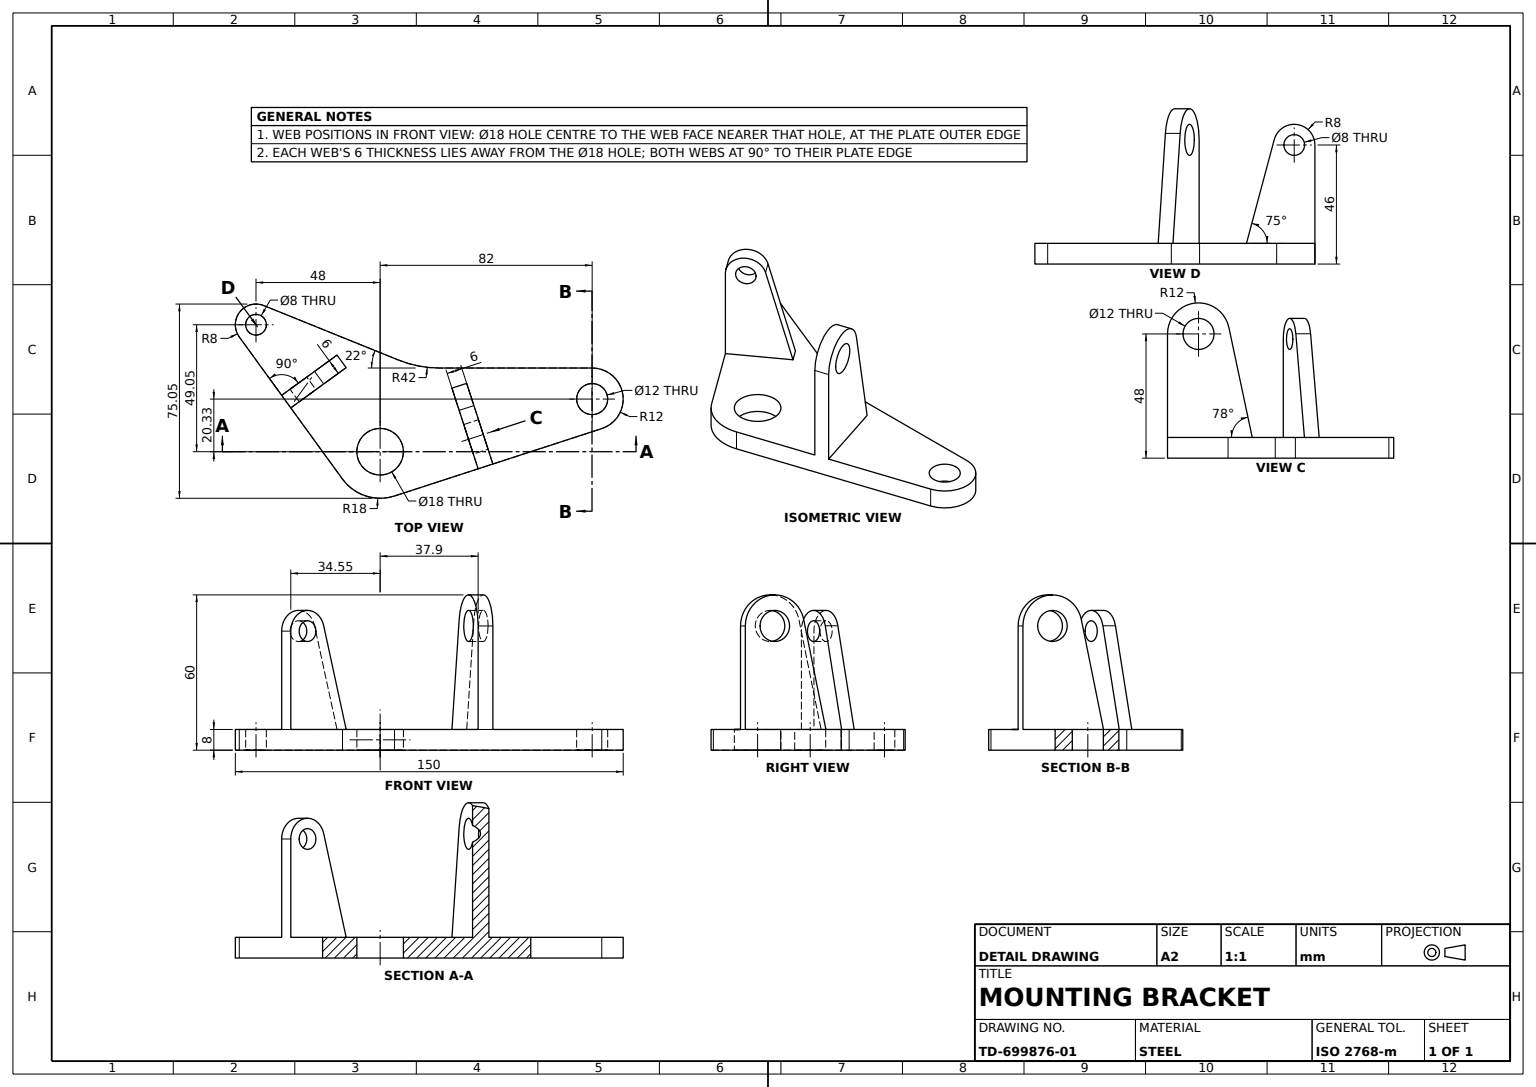
from build123d import *

# Parameters (mm, degrees)
BASE_PLATE_SKETCH_R      = 9
BASE_PLATE_SKETCH_R_2    = 6
BASE_PLATE_SKETCH_R_3    = 4
BASE_PLATE_DEPTH         = 8
UPRIGHT_WEB_DEPTH        = 98
WEB_ANGLED_TRIM_SKETCH_R = 4
WEB_ANGLED_TRIM_DEPTH    = 98
PIVOT_LUG_SKETCH_R       = 6
PIVOT_LUG_DEPTH          = 6
LUG_CUT_SKETCH_R         = 6
LUG_CUT_DEPTH            = 16


with BuildPart() as part:
    # Base Plate Sketch → Base Plate (new body)
    with BuildSketch(Plane(origin=(0, 0, 0), x_dir=(1, 0, 0), z_dir=(0, 1, 0))):
        with BuildLine():
            Line((82, 32.334641746), (22.899881176, 32.334641746))
            ThreePointArc((22.899881176, 32.334641746), (14.88590337, 33.106300041), (7.166404253, 35.392919854))
            Line((7.166404253, 35.392919854), (-45.003147253, 56.470786852))
            ThreePointArc((-45.003147253, 56.470786852), (-54.304086029, 53.978607818), (-54.472135955, 44.351033997))
            Line((-54.472135955, 44.351033997), (-14.562305899, -10.580134541))
            ThreePointArc((-14.562305899, -10.580134541), (-5.562305899, -17.119017293), (5.562305899, -17.119017293))
            Line((5.562305899, -17.119017293), (85.708203932, 8.92196355))
            ThreePointArc((85.708203932, 8.92196355), (93.852260087, 22.211855326), (82, 32.334641746))
        make_face()
        with Locations(Location((0, 0, 0), (0, 0, 270))):
            Circle(BASE_PLATE_SKETCH_R, mode=Mode.SUBTRACT)
        with Locations(Location((82, 20.334641746, 0), (0, 0, 270))):
            Circle(BASE_PLATE_SKETCH_R_2, mode=Mode.SUBTRACT)
        with Locations(Location((-48, 49.053316016, 0), (0, 0, 270))):
            Circle(BASE_PLATE_SKETCH_R_3, mode=Mode.SUBTRACT)
    extrude(amount=BASE_PLATE_DEPTH)

    # Upright Web Sketch → Upright Web (add)
    with BuildSketch(Plane(origin=(0, 8, 0), x_dir=(1, 0, 0), z_dir=(0, 1, 0))):
        Polygon((-34.547004477, 16.926443267), (-10.806972302, 34.174586259), (-14.333683815, 39.028688225), (-38.07371599, 21.780545234), align=None)
        Polygon((37.898227453, -6.612439485), (28.456105239, 22.447424608), (34.162444337, 24.301526574), (43.604566551, -4.758337518), align=None)
    extrude(amount=UPRIGHT_WEB_DEPTH)

    # Web Angled Trim Sketch → Web Angled Trim (cut)
    with BuildSketch(Plane(origin=(-23.511410092, 0, -32.360679775), x_dir=(-0.8090169943749421, 0, 0.5877852522924805), z_dir=(-0.5877852522924805, 0, -0.8090169943749422))):
        with Locations((10, 46)):
            Circle(WEB_ANGLED_TRIM_SKETCH_R)
        with BuildLine():
            Line((-8.464278756, 8), (2.27259339, 48.070552361))
            ThreePointArc((2.27259339, 48.070552361), (11.044209538, 53.931558891), (18, 46))
            Line((18, 46), (24.045319571, 43.356543138))
            Line((24.045319571, 43.356543138), (48.419235534, 110.549500658))
            Line((48.419235534, 110.549500658), (-18.279656122, 110.549500658))
            Line((-18.279656122, 110.549500658), (-16.138704045, 8))
            Line((-16.138704045, 8), (-8.464278756, 8))
        make_face()
    extrude(amount=-WEB_ANGLED_TRIM_DEPTH, mode=Mode.SUBTRACT)

    # Pivot Lug Sketch → Pivot Lug (add)
    with BuildSketch(Plane(origin=(38.042260652, 0, -12.360679775), x_dir=(-0.3090169943749489, 0, -0.9510565162951532), z_dir=(0.9510565162951532, 0, -0.3090169943749489))):
        with BuildLine():
            Line((14.770349605, 8), (5.737771209, 50.49494029))
            ThreePointArc((5.737771209, 50.49494029), (-7.254341559, 59.934262744), (-18, 48))
            Line((-18, 48), (-18, 8))
            Line((-18, 8), (14.770349605, 8))
        make_face()
        with Locations((-6, 48)):
            Circle(PIVOT_LUG_SKETCH_R, mode=Mode.SUBTRACT)
    extrude(amount=-PIVOT_LUG_DEPTH)

    # Lug Cut Sketch → Lug Cut (cut)
    with BuildSketch(Plane(origin=(38.042260652, 0, -12.360679775), x_dir=(-0.3090169943749489, 0, -0.9510565162951532), z_dir=(0.9510565162951532, 0, -0.3090169943749489))):
        with Locations((-6, 48)):
            Circle(LUG_CUT_SKETCH_R)
        with BuildLine():
            Line((12.555349334, 18.420756966), (5.737771209, 50.49494029))
            ThreePointArc((5.737771209, 50.49494029), (-7.254341559, 59.934262744), (-18, 48))
            Line((-18, 48), (-46.797997281, 119.82194568))
            Line((-46.797997281, 119.82194568), (32.722077442, 114.455560269))
            Line((32.722077442, 114.455560269), (12.555349334, 18.420756966))
        make_face()
    extrude(amount=-LUG_CUT_DEPTH, mode=Mode.SUBTRACT)


solid = part.part
